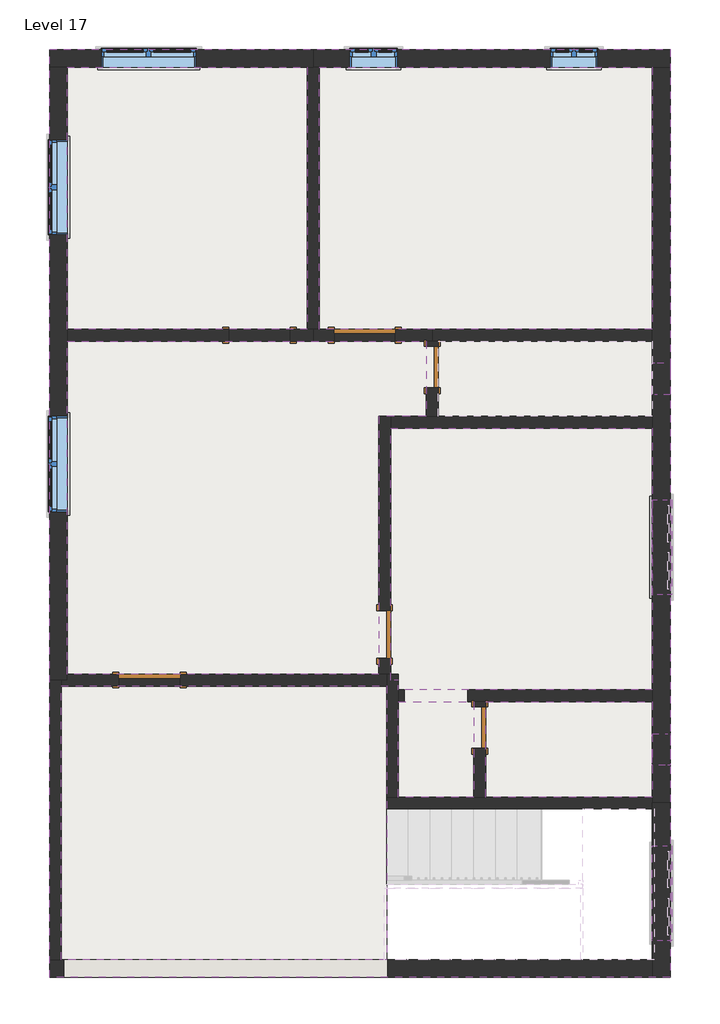
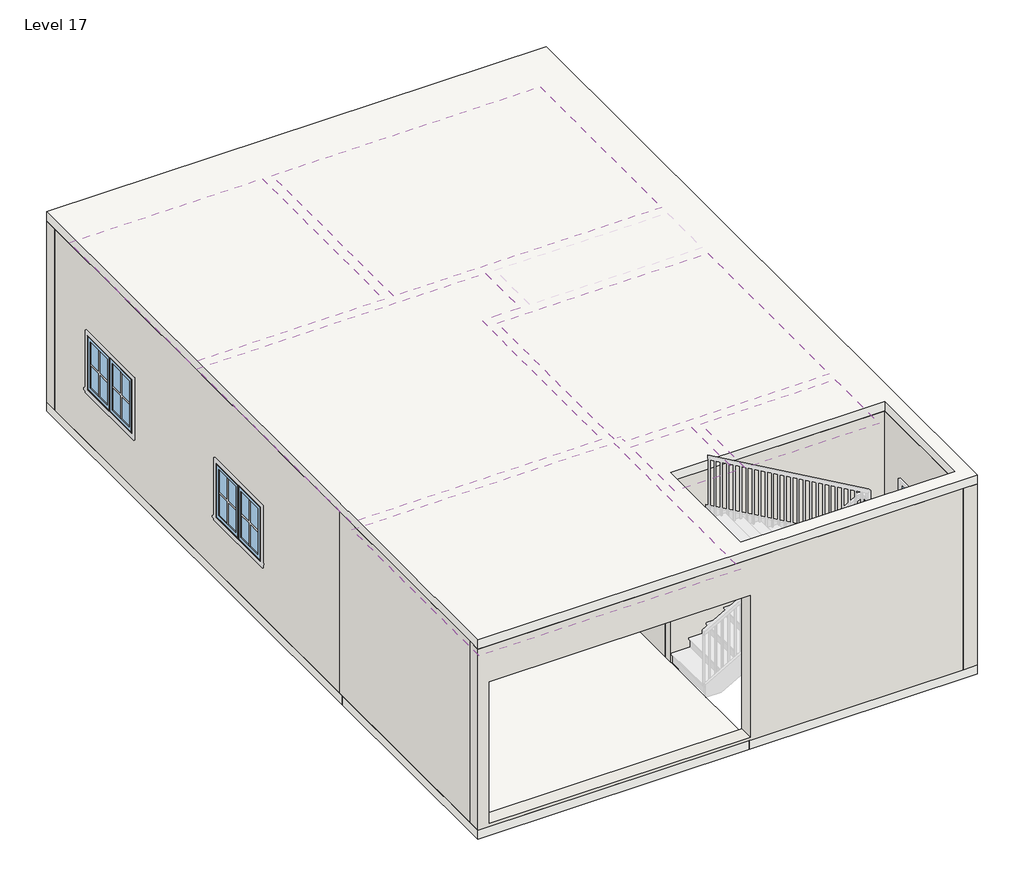
# One storey, part 1 of 2: 27 walls, 13 windows, 7 coverings, 6 doors, 3 slabs.
# Revit data of these elements (continued)
# Element 47 (IfcWindow, "Window-Casement-Double : 3'") (continued)
#   Materials on its faces: "Wood - Stained", "Glass", "Clad - White"
# Element 48 (IfcWindow, "Window-Casement-Double : 3'")
#   Mark = "64"
#   Window Inset = 0' - 0"
#   Interior Wall Closure = 0' - 2 1/4"
#   Frame Extension = 0' - 0 1/4"
#   Exterior Wall Closure = 0' - 1 1/4"
#   Interior Trim Visibility = yes
#   Exterior Trim Visibility = yes
#   Phase Created = New Construction
#   Materials on its faces: "Wood - Stained", "Glass", "Clad - White"
# Element 49 (IfcWindow, "Window-Casement-Double : 3'")
#   Mark = "65"
#   Window Inset = 0' - 0"
#   Interior Wall Closure = 0' - 2 1/4"
#   Frame Extension = 0' - 0 1/4"
#   Exterior Wall Closure = 0' - 1 1/4"
#   Interior Trim Visibility = yes
#   Exterior Trim Visibility = yes
#   Phase Created = New Construction
#   Materials on its faces: "Wood - Stained", "Glass", "Clad - White"
# Element 50 (IfcWindow, "Window-Casement-Double : 4'")
#   Mark = "53"
#   Window Inset = 0' - 0"
#   Interior Wall Closure = 0' - 2 1/4"
#   Frame Extension = 0' - 0 1/4"
#   Exterior Wall Closure = 0' - 1 1/4"
#   Interior Trim Visibility = yes
#   Exterior Trim Visibility = yes
#   Phase Created = New Construction
#   Materials on its faces: "Wood - Stained", "Glass", "Clad - White"
# Element 51 (IfcWindow, "Window-Casement-Double : 4'")
#   Mark = "54"
#   Window Inset = 0' - 0"
#   Interior Wall Closure = 0' - 2 1/4"
#   Frame Extension = 0' - 0 1/4"
#   Exterior Wall Closure = 0' - 1 1/4"
#   Interior Trim Visibility = yes
#   Exterior Trim Visibility = yes
#   Phase Created = New Construction
#   Materials on its faces: "Wood - Stained", "Glass", "Clad - White"
# Element 52 (IfcWindow, "Window-Casement-Double : 4'")
#   Mark = "55"
#   Window Inset = 0' - 0"
#   Interior Wall Closure = 0' - 2 1/4"
#   Frame Extension = 0' - 0 1/4"
#   Exterior Wall Closure = 0' - 1 1/4"
#   Interior Trim Visibility = yes
#   Exterior Trim Visibility = yes
#   Phase Created = New Construction
#   Materials on its faces: "Wood - Stained", "Glass", "Clad - White"
# Element 53 (IfcWindow, "Window-Casement-Double : 4'")
#   Mark = "56"
#   Window Inset = 0' - 0"
#   Interior Wall Closure = 0' - 2 1/4"
#   Frame Extension = 0' - 0 1/4"
#   Exterior Wall Closure = 0' - 1 1/4"
#   Interior Trim Visibility = yes
#   Exterior Trim Visibility = yes
#   Phase Created = New Construction
#   Materials on its faces: "Wood - Stained", "Glass", "Clad - White"
# Element 54 (IfcWindow, "Window-Casement-Double : 4'")
#   Mark = "57"
#   Window Inset = 0' - 0"
#   Interior Wall Closure = 0' - 2 1/4"
#   Frame Extension = 0' - 0 1/4"
#   Exterior Wall Closure = 0' - 1 1/4"
#   Interior Trim Visibility = yes
#   Exterior Trim Visibility = yes
#   Phase Created = New Construction
#   Materials on its faces: "Wood - Stained", "Glass", "Clad - White"
# Element 55 (IfcWindow, "Window-Casement-Double : 4'")
#   Mark = "62"
#   Window Inset = 0' - 0"
#   Interior Wall Closure = 0' - 2 1/4"
#   Frame Extension = 0' - 0 1/4"
#   Exterior Wall Closure = 0' - 1 1/4"
#   Interior Trim Visibility = yes
#   Exterior Trim Visibility = yes
#   Phase Created = New Construction
#   Materials on its faces: "Wood - Stained", "Glass", "Clad - White"
# Element 56 (IfcWindow, "Window-Casement-Double : 4'")
#   Mark = "63"
#   Window Inset = 0' - 0"
#   Interior Wall Closure = 0' - 2 1/4"
#   Frame Extension = 0' - 0 1/4"
#   Exterior Wall Closure = 0' - 1 1/4"
#   Interior Trim Visibility = yes
#   Exterior Trim Visibility = yes
#   Phase Created = New Construction
#   Materials on its faces: "Wood - Stained", "Glass", "Clad - White"
# Materials
#   "Default": colour RGB 127 127 127, transparency 0, Cost = 0
#   "Acoustic Ceiling Tile 24 x 48": class "Generic", colour RGB 229 229 229, transparency 0, Description = "Acoustic Ceiling Tile 24 x 48", Cost = 0
#   "Door - Panel": class "Wood", colour RGB 210 159 95, transparency 0, Cost = 0
#   "Door - Frame": colour RGB 118 70 51, transparency 0, Cost = 0
#   "Glass": class "Glass", colour RGB 0 128 192, transparency 0.75, Description = "Soda Lime Glass", Cost = 0
#   "Sash": class "Wood", colour RGB 224 178 126, transparency 0, Cost = 0
#   "Wood - Stained": class "Wood", colour RGB 224 178 126, transparency 0, Cost = 0
#   "Clad - White": class "Wood", colour RGB 242 242 238, transparency 0, Cost = 0
#   "Default Floor": colour RGB 128 128 128, transparency 0, Cost = 0
#   "TILE": class "Generic", colour RGB 120 120 120, transparency 0, Cost = 0
#   "Grass": class "Generic", colour RGB 104 137 66, transparency 0, Description = "Physical material.", Cost = 0
#   "Default Wall": colour RGB 128 128 128, transparency 0, Cost = 0
#   "WALL PAINT 4": class "Generic", colour RGB 120 120 120, transparency 0, Cost = 0
#   "MARBLE": class "Generic", colour RGB 120 120 120, transparency 0, Cost = 0
#   "WALL PAINT 5": class "Generic", colour RGB 120 120 120, transparency 0, Cost = 0
#   "WALL PAINT 2": class "Generic", colour RGB 120 120 120, transparency 0, Cost = 0
#   "WALL PAINT 3": class "Generic", colour RGB 120 120 120, transparency 0, Cost = 0
#   "WALL PAINT 1": class "Generic", colour RGB 120 120 120, transparency 0, Cost = 0
